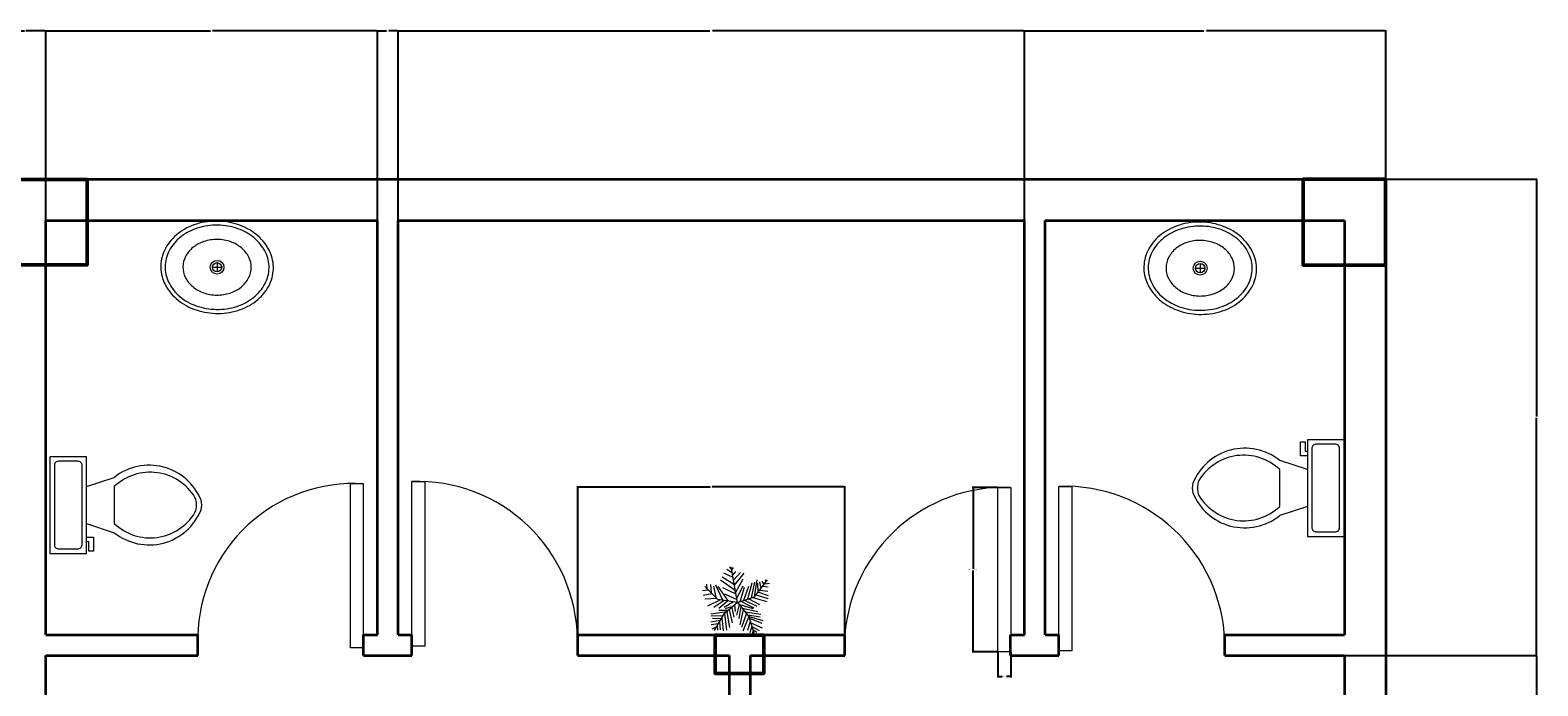
# Model space of a CAD drawing. Units: inches. Extents: x 50 to 2003, y -28 to 675.
# Tile 4 of 10: x 218 to 545, y 532 to 675. Entities that reach past the tile are written whole.
import ezdxf

# ---------------------------------------------------------------- set-up
doc = ezdxf.new("R2010")
doc.units = ezdxf.units.IN
for name, color, linetype, lineweight in [('A-ANNO-DIMS', 2, 'Continuous', 18), ('A-COLS', 1, 'Continuous', 50), ('A-DOOR', 4, 'Continuous', 18), ('A-FLOR-FIXT', 9, 'Continuous', 18), ('A-WALL', 7, 'Continuous', 35), ('L-PLNT', 3, 'Continuous', 13)]:
    doc.layers.add(name, color=color, linetype=linetype, lineweight=lineweight)
doc.styles.get("Standard").update_dxf_attribs({"font": 'arial.ttf'})
doc.dimstyles.get("Standard").update_dxf_attribs({"dimtxt": 0.18, "dimasz": 0.18, "dimexe": 0.18, "dimexo": 0.0625, "dimgap": 0.09, "dimtad": 0, "dimtih": 1, "dimtoh": 1, "dimdec": 4, "dimzin": 0, "dimdsep": 46, "dimtxsty": 'Standard', "dimcen": 0.09, "dimadec": 0, "dimazin": 0, "dimtfac": 1, "dimtdec": 4, "dimtofl": 0, "dimtmove": 0, "dimatfit": 3, "dimfxl": 1, "dimtolj": 1, "dimtzin": 0, "dimarcsym": 0})

# ---------------------------------------------------------------- blocks, each defined once
blk = doc.blocks.new('*U2')
for p, q in [((-8.737, 47.138), (-17.069, 52.711)), ((-10.186, 53.64), (-13.084, 55.962)), ((0, 0), (-10.5, 57)), ((-9.099, 51.782), (-6.563, 55.962)), ((-7.65, 43.423), (-2.578, 49.46)), ((-31.5, 4.5), (-52.5, 25.5)), ((-48.585, 21.131), (-49.309, 29.026)), ((-43.513, 28.561), (-42.427, 15.558)), ((-38.442, 26.239), (-34.819, 7.663)), ((-35.544, 28.097), (-24.314, 3.947)), ((-14.533, 2.09), (-30.834, 25.31)), ((-3.665, 19.273), (-27.574, 35.527)), ((-5.114, 28.097), (-24.676, 40.636)), ((-7.288, 39.707), (-21.778, 46.673)), ((-5.839, 35.992), (4.667, 48.067)), ((-5.114, 27.632), (10.463, 46.673)), ((-2.941, 16.486), (8.652, 37.85)), ((-1.129, 6.734), (9.014, 26.704)), ((3.942, 1.625), (11.187, 24.381)), ((10.101, 3.483), (17.708, 26.239)), ((16.259, 5.805), (23.142, 31.348)), ((22.055, 7.198), (27.489, 32.277)), ((27, 9), (48, 36)), ((27.127, 9.056), (31.112, 35.992)), ((31.836, 30.883), (32.561, 16.486)), ((35.096, 32.741), (37.27, 22.524)), ((38.719, 34.134), (41.979, 28.561)), ((40.53, 25.775), (48.862, 24.846)), ((43.791, 29.954), (51.036, 30.883)), ((44.153, 36.456), (45.239, 32.741)), ((-47.498, 19.737), (-55.83, 18.344)), ((-40.615, 13.7), (-55.105, 10.913)), ((-33.37, 6.269), (-52.207, 5.34)), ((-28.299, 3.483), (-47.86, -5.805)), ((-21.416, 3.018), (-38.079, -8.128)), ((0, 0), (-31.5, 4.5)), ((-15.982, 2.09), (-30.11, -9.521)), ((-24.314, 23.917), (-2.941, 13.7)), ((0, 0), (-22.5, -19.5)), ((-6.563, 1.161), (-21.416, -8.128)), ((-20.691, 13.7), (-1.129, 4.876)), ((0, 0), (27, 9)), ((0, 0), (18, -22.5)), ((6.478, 1.625), (26.04, -8.592)), ((11.187, 3.483), (30.749, -5.805)), ((18.07, 5.805), (35.096, -3.483)), ((24.229, 7.663), (46.688, 1.625)), ((29.662, 12.307), (48.137, 6.269)), ((33.285, 16.486), (48.862, 10.913)), ((36.183, 19.737), (48.137, 17.88)), ((-17.431, -15.094), (-42.789, -18.809)), ((-24.314, -21.596), (-42.427, -22.06)), ((-22.5, -19.5), (-37.5, -45)), ((-15.257, -12.772), (-30.11, -12.772)), ((-25.038, -23.918), (-22.865, -45.281)), ((-20.691, -18.345), (-17.793, -44.352)), ((-6.563, -5.805), (-19.967, -9.985)), ((-17.069, -15.094), (-12.721, -40.172)), ((-13.446, -11.378), (-8.737, -32.741)), ((-9.461, -8.592), (-6.201, -23.453)), ((-4.752, -3.483), (-3.665, -14.629)), ((2.493, -3.019), (-1.491, -20.202)), ((1.769, -2.555), (24.229, -9.521)), ((5.029, -6.27), (2.131, -25.775)), ((9.014, -11.378), (3.58, -35.992)), ((14.085, -16.951), (6.478, -40.172)), ((7.565, -9.056), (32.198, -14.629)), ((18.07, -22.524), (8.289, -45.745)), ((12.274, -15.094), (36.907, -18.809)), ((16.259, -19.738), (36.183, -22.989)), ((18, -22.5), (27, -52.5)), ((18.433, -22.524), (40.53, -29.026)), ((-28.299, -29.026), (-42.789, -31.348)), ((-30.834, -34.135), (-42.427, -35.528)), ((-34.457, -39.708), (-40.978, -42.494)), ((-26.849, -26.24), (-40.253, -25.775)), ((-32.646, -36.921), (-31.921, -44.352)), ((-29.023, -30.884), (-27.936, -43.887)), ((20.244, -30.419), (15.897, -44.816)), ((19.157, -25.311), (38.719, -33.206)), ((22.78, -37.85), (19.519, -48.532)), ((21.331, -32.741), (39.081, -40.636)), ((22.78, -38.314), (34.372, -44.816)), ((24.591, -45.745), (23.142, -50.854)), ((24.591, -43.423), (30.749, -47.603)), ((26.764, -49.925), (28.213, -50.854))]:
    blk.add_line(p, q)
blk = doc.blocks.new('Toilet - top')
for p, q in [((9.5, -6), (9.5, -2)), ((-10, -8.5), (-8, -8.5)), ((-10, -9.5), (-10, -8.5)), ((-7, -9.5), (-10, -9.5)), ((-8, -8.5), (-8, -8)), ((-7, -8), (-7, -9.5)), ((-4, -8), (-6, -14)), ((4, -8), (6, -14)), ((4, -14), (-4, -14))]:
    blk.add_line(p, q)
blk.add_lwpolyline([(10.5, -8), (10.5, 0), (-10.5, 0), (-10.5, -8)], close=True)
for points in [[(-9.5, -2), (-9.5, -6)], [(8.5, -1), (-8.5, -1)], [(-8.5, -7), (8.5, -7)]]:
    blk.add_lwpolyline(points)
for centre, radius, start, end in [((-8.62, -1.88), 0.884, 81.8699, 188.1301), ((8.62, -1.88), 0.884, 351.8699, 98.1301), ((-8.62, -6.12), 0.884, 171.8699, 278.1301), ((8.62, -6.12), 0.884, 261.8699, 8.1301), ((3.52, -21.58), 12.17, 141.4691, 247.9714), ((4.2, -21.82), 11.33, 136.3677, 238.9468), ((-3.52, -21.58), 12.17, 292.0284, 38.5307), ((-4.2, -21.82), 11.33, 301.053, 43.6321), ((0, -27.88), 4, 245.7318, 294.2682), ((0, -29), 4, 254.8605, 285.1395)]:
    blk.add_arc(centre, radius, start, end)
blk = doc.blocks.new('Sink - Oval top')
for p, q in [((-1, 0), (1, 0)), ((0, 1), (0, -1))]:
    blk.add_line(p, q)
for points in [[(-12.23, 0.39, 0.117634), (-11.46, -3.36, 0.104469), (-8.88, -6.8, 0.090016), (-5.08, -9.07, 0.08192), (-0.32, -10.02, 0.08192), (4.49, -9.38, 0.090016), (8.42, -7.36, 0.104469), (11.22, -4.09, 0.117634), (12.23, -0.39, 0.117634), (11.46, 3.36, 0.104469), (8.88, 6.8, 0.090016), (5.08, 9.07, 0.08192), (0.32, 10.02, 0.08192), (-4.49, 9.38, 0.090016), (-8.42, 7.36, 0.104469), (-11.22, 4.09, 0.117634)], [(-11.29, 0.16, 0.118622), (-10.52, -3.25, 0.104678), (-8.07, -6.36, 0.089562), (-4.54, -8.37, 0.081185), (-0.13, -9.15, 0.081185), (4.3, -8.49, 0.089562), (7.89, -6.58, 0.104678), (10.42, -3.55, 0.118622), (11.29, -0.16, 0.118622), (10.52, 3.25, 0.104678), (8.07, 6.36, 0.089562), (4.54, 8.37, 0.081185), (0.13, 9.15, 0.081185), (-4.3, 8.49, 0.089562), (-7.89, 6.58, 0.104678), (-10.42, 3.55, 0.118622)], [(-7.42, 0.08, 0.118283), (-6.91, -2.17, 0.104607), (-5.29, -4.21, 0.089718), (-2.97, -5.53, 0.081436), (-0.07, -6.04, 0.081436), (2.84, -5.59, 0.089718), (5.2, -4.33, 0.104607), (6.86, -2.32, 0.118283), (7.42, -0.08, 0.118283), (6.91, 2.17, 0.104607), (5.29, 4.21, 0.089718), (2.97, 5.53, 0.081436), (0.07, 6.04, 0.081436), (-2.84, 5.59, 0.089718), (-5.2, 4.33, 0.104607), (-6.86, 2.32, 0.118283)]]:
    blk.add_lwpolyline(points, format="xyb", close=True)
for radius in [1.5, 1]:
    blk.add_circle((0, 0), radius)
blk = doc.blocks.new('DOOR-LEAF-36')
blk.add_lwpolyline([(35.71, 2.81), (35.71, 0), (0, 0), (0, 2.81)], close=True)
blk = doc.blocks.new('*D21')
at = {"layer": 'A-ANNO-DIMS', "color": 0, "lineweight": -2, "transparency": 16777216}
for p, q in [((427.62, 575.33), (422.15, 575.33)), ((422.33, 575.15), (422.33, 557.66)), ((422.33, 539.81), (422.33, 557.3)), ((427.62, 539.63), (422.15, 539.63))]:
    blk.add_line(p, q, dxfattribs=at)
at = {"layer": 'A-ANNO-DIMS', "color": 0, "transparency": 16777216}
for points in [[(422.3, 575.15), (422.36, 575.15), (422.33, 575.33)], [(422.3, 539.81), (422.36, 539.81), (422.33, 539.63)]]:
    blk.add_solid(points, dxfattribs=at)
at = {"layer": 'Defpoints', "color": 0, "transparency": 16777216}
for p in [(427.69, 575.33), (422.33, 539.63), (427.69, 539.63)]:
    blk.add_point(p, dxfattribs=at)
at = {"layer": 'A-ANNO-DIMS', "color": 0, "transparency": 16777216, "insert": (422.33, 557.48), "char_height": 0.18, "attachment_point": 5}
blk.add_mtext('\\A1;DOOR LEAF 36 TYP.', dxfattribs=at)
blk = doc.blocks.new('*D22')
at = {"layer": 'A-ANNO-DIMS', "color": 0, "lineweight": -2, "transparency": 16777216}
for p, q in [((427.69, 539.56), (427.69, 534.09)), ((430.5, 539.56), (430.5, 534.09)), ((427.87, 534.27), (428.63, 534.27)), ((430.32, 534.27), (429.55, 534.27))]:
    blk.add_line(p, q, dxfattribs=at)
at = {"layer": 'A-ANNO-DIMS', "color": 0, "transparency": 16777216}
for points in [[(427.87, 534.3), (427.87, 534.24), (427.69, 534.27)], [(430.32, 534.3), (430.32, 534.24), (430.5, 534.27)]]:
    blk.add_solid(points, dxfattribs=at)
at = {"layer": 'Defpoints', "color": 0, "transparency": 16777216}
for p in [(427.69, 539.63), (430.5, 539.63), (430.5, 534.27)]:
    blk.add_point(p, dxfattribs=at)
at = {"layer": 'A-ANNO-DIMS', "color": 0, "transparency": 16777216, "insert": (429.09, 534.27), "char_height": 0.18, "attachment_point": 5}
blk.add_mtext('\\A1;3 TYP.', dxfattribs=at)
blk = doc.blocks.new('*D54')
at = {"layer": 'A-ANNO-DIMS', "color": 0, "lineweight": -2, "transparency": 16777216}
for p, q in [((211.97, 642.39), (211.97, 674.65)), ((212.15, 674.47), (216.32, 674.47)), ((220.79, 674.47), (216.62, 674.47)), ((220.97, 633.39), (220.97, 674.65))]:
    blk.add_line(p, q, dxfattribs=at)
at = {"layer": 'A-ANNO-DIMS', "color": 0, "transparency": 16777216}
for points in [[(212.15, 674.5), (212.15, 674.44), (211.97, 674.47)], [(220.79, 674.5), (220.79, 674.44), (220.97, 674.47)]]:
    blk.add_solid(points, dxfattribs=at)
at = {"layer": 'Defpoints', "color": 0, "transparency": 16777216}
for p in [(220.97, 674.47), (211.97, 642.32), (220.97, 633.32)]:
    blk.add_point(p, dxfattribs=at)
at = {"layer": 'A-ANNO-DIMS', "color": 0, "transparency": 16777216, "insert": (216.47, 674.47), "char_height": 0.18, "attachment_point": 5}
blk.add_mtext('\\A1;9', dxfattribs=at)
blk = doc.blocks.new('*D55')
at = {"layer": 'A-ANNO-DIMS', "color": 0, "lineweight": -2, "transparency": 16777216}
for p, q in [((220.97, 633.39), (220.97, 674.65)), ((221.15, 674.47), (256.75, 674.47)), ((292.79, 674.47), (257.19, 674.47)), ((292.97, 633.39), (292.97, 674.65))]:
    blk.add_line(p, q, dxfattribs=at)
at = {"layer": 'A-ANNO-DIMS', "color": 0, "transparency": 16777216}
for points in [[(221.15, 674.5), (221.15, 674.44), (220.97, 674.47)], [(292.79, 674.5), (292.79, 674.44), (292.97, 674.47)]]:
    blk.add_solid(points, dxfattribs=at)
at = {"layer": 'Defpoints', "color": 0, "transparency": 16777216}
for p in [(292.97, 674.47), (220.97, 633.32), (292.97, 633.32)]:
    blk.add_point(p, dxfattribs=at)
at = {"layer": 'A-ANNO-DIMS', "color": 0, "transparency": 16777216, "insert": (256.97, 674.47), "char_height": 0.18, "attachment_point": 5}
blk.add_mtext('\\A1;72', dxfattribs=at)
blk = doc.blocks.new('*D56')
at = {"layer": 'A-ANNO-DIMS', "color": 0, "lineweight": -2, "transparency": 16777216}
for p, q in [((292.97, 633.39), (292.97, 674.65)), ((293.15, 674.47), (294.96, 674.47)), ((297.29, 674.47), (295.48, 674.47)), ((297.47, 633.39), (297.47, 674.65))]:
    blk.add_line(p, q, dxfattribs=at)
at = {"layer": 'A-ANNO-DIMS', "color": 0, "transparency": 16777216}
for points in [[(293.15, 674.5), (293.15, 674.44), (292.97, 674.47)], [(297.29, 674.5), (297.29, 674.44), (297.47, 674.47)]]:
    blk.add_solid(points, dxfattribs=at)
at = {"layer": 'Defpoints', "color": 0, "transparency": 16777216}
for p in [(297.47, 674.47), (292.97, 633.32), (297.47, 633.32)]:
    blk.add_point(p, dxfattribs=at)
at = {"layer": 'A-ANNO-DIMS', "color": 0, "transparency": 16777216, "insert": (295.22, 674.47), "char_height": 0.18, "attachment_point": 5}
blk.add_mtext('\\A1;4.5', dxfattribs=at)
blk = doc.blocks.new('*D57')
at = {"layer": 'A-ANNO-DIMS', "color": 0, "lineweight": -2, "transparency": 16777216}
for p, q in [((297.47, 633.39), (297.47, 674.65)), ((297.65, 674.47), (365.19, 674.47)), ((433.29, 674.47), (365.75, 674.47)), ((433.47, 633.39), (433.47, 674.65))]:
    blk.add_line(p, q, dxfattribs=at)
at = {"layer": 'A-ANNO-DIMS', "color": 0, "transparency": 16777216}
for points in [[(297.65, 674.5), (297.65, 674.44), (297.47, 674.47)], [(433.29, 674.5), (433.29, 674.44), (433.47, 674.47)]]:
    blk.add_solid(points, dxfattribs=at)
at = {"layer": 'Defpoints', "color": 0, "transparency": 16777216}
for p in [(433.47, 674.47), (297.47, 633.32), (433.47, 633.32)]:
    blk.add_point(p, dxfattribs=at)
at = {"layer": 'A-ANNO-DIMS', "color": 0, "transparency": 16777216, "insert": (365.47, 674.47), "char_height": 0.18, "attachment_point": 5}
blk.add_mtext('\\A1;136', dxfattribs=at)
blk = doc.blocks.new('*D58')
at = {"layer": 'A-ANNO-DIMS', "color": 0, "lineweight": -2, "transparency": 16777216}
for p, q in [((433.47, 633.39), (433.47, 674.65)), ((433.65, 674.47), (472.4, 674.47)), ((511.79, 674.47), (473.04, 674.47)), ((511.97, 642.39), (511.97, 674.65))]:
    blk.add_line(p, q, dxfattribs=at)
at = {"layer": 'A-ANNO-DIMS', "color": 0, "transparency": 16777216}
for points in [[(433.65, 674.5), (433.65, 674.44), (433.47, 674.47)], [(511.79, 674.5), (511.79, 674.44), (511.97, 674.47)]]:
    blk.add_solid(points, dxfattribs=at)
at = {"layer": 'Defpoints', "color": 0, "transparency": 16777216}
for p in [(511.97, 674.47), (511.97, 642.32), (433.47, 633.32)]:
    blk.add_point(p, dxfattribs=at)
at = {"layer": 'A-ANNO-DIMS', "color": 0, "transparency": 16777216, "insert": (472.72, 674.47), "char_height": 0.18, "attachment_point": 5}
blk.add_mtext('\\A1;78.5', dxfattribs=at)
blk = doc.blocks.new('*D62')
at = {"layer": 'A-ANNO-DIMS', "color": 0, "lineweight": -2, "transparency": 16777216}
for p, q in [((503.03, 538.82), (544.84, 538.82)), ((544.66, 538.64), (544.66, 465.26)), ((544.66, 391.5), (544.66, 464.89)), ((503.03, 391.32), (544.84, 391.32))]:
    blk.add_line(p, q, dxfattribs=at)
at = {"layer": 'A-ANNO-DIMS', "color": 0, "transparency": 16777216}
for points in [[(544.63, 538.64), (544.69, 538.64), (544.66, 538.82)], [(544.63, 391.5), (544.69, 391.5), (544.66, 391.32)]]:
    blk.add_solid(points, dxfattribs=at)
at = {"layer": 'Defpoints', "color": 0, "transparency": 16777216}
for p in [(502.97, 538.82), (544.66, 538.82), (502.97, 391.32)]:
    blk.add_point(p, dxfattribs=at)
at = {"layer": 'A-ANNO-DIMS', "color": 0, "transparency": 16777216, "insert": (544.66, 465.07), "char_height": 0.18, "attachment_point": 5}
blk.add_mtext('\\A1;147.5', dxfattribs=at)
blk = doc.blocks.new('*D63')
at = {"layer": 'A-ANNO-DIMS', "color": 0, "lineweight": -2, "transparency": 16777216}
for p, q in [((512.03, 642.32), (544.84, 642.32)), ((544.66, 642.14), (544.66, 590.76)), ((544.66, 539), (544.66, 590.39)), ((503.03, 538.82), (544.84, 538.82))]:
    blk.add_line(p, q, dxfattribs=at)
at = {"layer": 'A-ANNO-DIMS', "color": 0, "transparency": 16777216}
for points in [[(544.63, 642.14), (544.69, 642.14), (544.66, 642.32)], [(544.63, 539), (544.69, 539), (544.66, 538.82)]]:
    blk.add_solid(points, dxfattribs=at)
at = {"layer": 'Defpoints', "color": 0, "transparency": 16777216}
for p in [(511.97, 642.32), (544.66, 642.32), (502.97, 538.82)]:
    blk.add_point(p, dxfattribs=at)
at = {"layer": 'A-ANNO-DIMS', "color": 0, "transparency": 16777216, "insert": (544.66, 590.57), "char_height": 0.18, "attachment_point": 5}
blk.add_mtext('\\A1;103.5', dxfattribs=at)
blk = doc.blocks.new('*D69')
at = {"layer": 'A-ANNO-DIMS', "color": 0, "lineweight": -2, "transparency": 16777216}
for p, q in [((336.47, 543.39), (336.47, 575.65)), ((336.65, 575.47), (365.25, 575.47)), ((394.29, 575.47), (365.69, 575.47)), ((394.47, 543.39), (394.47, 575.65))]:
    blk.add_line(p, q, dxfattribs=at)
at = {"layer": 'A-ANNO-DIMS', "color": 0, "transparency": 16777216}
for points in [[(336.65, 575.5), (336.65, 575.44), (336.47, 575.47)], [(394.29, 575.5), (394.29, 575.44), (394.47, 575.47)]]:
    blk.add_solid(points, dxfattribs=at)
at = {"layer": 'Defpoints', "color": 0, "transparency": 16777216}
for p in [(394.47, 575.47), (336.47, 543.32), (394.47, 543.32)]:
    blk.add_point(p, dxfattribs=at)
at = {"layer": 'A-ANNO-DIMS', "color": 0, "transparency": 16777216, "insert": (365.47, 575.47), "char_height": 0.18, "attachment_point": 5}
blk.add_mtext('\\A1;58', dxfattribs=at)

msp = doc.modelspace()

# ---------------------------------------------------------------- linework, layer by layer
at = {"layer": 'A-COLS'}
for points in [[(211.9898, 642.1898), (229.9336, 642.1898), (229.9336, 623.6596), (211.9898, 623.6596)], [(511.9071, 642.2546), (493.9902, 642.2546), (493.9902, 623.6344), (511.9071, 623.6344)], [(366.2895, 543.2564), (376.8583, 543.2564), (376.8583, 534.9486), (366.2895, 534.9486)]]:
    msp.add_lwpolyline(points, close=True, dxfattribs=at)
at = {"layer": 'A-DOOR'}
for centre, radius, start, end in [((287.8796, 542.2862), 33.9113, 86.591193, 178.879605), ((301.7332, 541.9614), 34.669, 0.787409, 92.068961), ((429.1629, 540.5706), 34.7894, 87.826126, 175.644292), ((442.1372, 540.7332), 34.8536, 1.948939, 91.91482)]:
    msp.add_arc(centre, radius, start, end, dxfattribs=at)
at = {"layer": 'A-WALL'}
for p, q in [((211.9711, 642.3232), (511.9711, 642.3232)), ((511.9711, 642.3232), (511.9711, 17.3232)), ((220.9711, 633.3232), (292.9711, 633.3232)), ((220.9711, 543.3232), (220.9711, 633.3232)), ((292.9711, 543.3232), (292.9711, 633.3232)), ((297.4711, 543.3232), (297.4711, 633.3232)), ((297.4711, 633.3232), (433.4711, 633.3232)), ((433.4711, 543.3232), (433.4711, 633.3232)), ((437.9711, 543.3232), (437.9711, 633.3232)), ((437.9711, 633.3232), (502.9711, 633.3232)), ((502.9711, 633.3232), (502.9711, 543.3232)), ((220.9711, 543.3232), (253.9711, 543.3232)), ((253.9711, 538.8232), (253.9711, 543.3232)), ((289.9711, 538.8232), (289.9711, 543.3232)), ((289.9711, 543.3232), (292.9711, 543.3232)), ((297.4711, 543.3232), (300.4711, 543.3232)), ((300.4711, 538.8232), (300.4711, 543.3232)), ((336.4711, 538.8232), (336.4711, 543.3232)), ((336.4711, 543.3232), (394.4711, 543.3232)), ((394.4711, 538.8232), (394.4711, 543.3232)), ((430.4711, 538.8232), (430.4711, 543.3232)), ((430.4711, 543.3232), (433.4711, 543.3232)), ((437.9711, 543.3232), (440.9711, 543.3232)), ((440.9711, 538.8232), (440.9711, 543.3232)), ((476.9711, 538.8232), (476.9711, 543.3232)), ((476.9711, 543.3232), (502.9711, 543.3232)), ((220.9711, 538.8232), (253.9711, 538.8232)), ((220.9711, 395.8232), (220.9711, 538.8232)), ((289.9711, 538.8232), (300.4711, 538.8232)), ((336.4711, 538.8232), (369.4711, 538.8232)), ((369.4711, 395.8232), (369.4711, 538.8232)), ((373.9711, 395.8232), (373.9711, 538.8232)), ((373.9711, 538.8232), (394.4711, 538.8232)), ((430.4711, 538.8232), (440.9711, 538.8232)), ((476.9711, 538.8232), (502.9711, 538.8232)), ((502.9711, 538.8232), (502.9711, 395.8232))]:
    msp.add_line(p, q, dxfattribs=at)

# ---------------------------------------------------------------- block references
at = {"layer": 'A-DOOR'}
for p, rotation in [((300.4835, 576.6088), 269.9999999999999), ((287.1102, 576.1839), 269.9999999999999), ((427.6868, 575.3339), 269.9999999999998), ((440.9775, 575.5669), 269.9999999999998)]:
    msp.add_blockref('DOOR-LEAF-36', p, dxfattribs=dict(at, rotation=rotation))
at = {"layer": 'A-FLOR-FIXT'}
for p in [(258.1642, 623.1544), (471.6425, 622.9522)]:
    msp.add_blockref('Sink - Oval top', p, dxfattribs=at)
for p, rotation in [((502.9091, 575.2126), 270), ((221.8432, 571.5115), 89.99999999999999)]:
    msp.add_blockref('Toilet - top', p, dxfattribs=dict(at, rotation=rotation))
at = {"layer": 'L-PLNT', "xscale": 0.1358686367750108, "yscale": 0.1358686367750108, "zscale": 0.1358686367750108}
msp.add_blockref('*U2', (371.192, 550.3577), dxfattribs=at)

# ---------------------------------------------------------------- dimensions: what is measured, and where the dimension line sits
at = {"layer": 'A-ANNO-DIMS'}
for base, p1, p2, override, picture, middle in [((220.9711, 674.4732), (211.9711, 642.3232), (220.9711, 633.3232), {"dimdec": 0, "dimlfac": 1, "dimrnd": 0, "dimzin": 0, "dimdsep": 46, "dimlunit": 2}, '*D54', (216.4711, 674.4732)), ((292.9711, 674.4732), (220.9711, 633.3232), (292.9711, 633.3232), {"dimdec": 0, "dimlfac": 1, "dimrnd": 0, "dimzin": 0, "dimdsep": 46, "dimlunit": 2}, '*D55', (256.9711, 674.4732)), ((297.4711, 674.4732), (292.9711, 633.3232), (297.4711, 633.3232), {"dimdec": 1, "dimlfac": 1, "dimrnd": 0, "dimzin": 0, "dimdsep": 46, "dimlunit": 2}, '*D56', (295.2211, 674.4732)), ((433.4711, 674.4732), (297.4711, 633.3232), (433.4711, 633.3232), {"dimdec": 0, "dimlfac": 1, "dimrnd": 0, "dimzin": 0, "dimdsep": 46, "dimlunit": 2}, '*D57', (365.4711, 674.4732)), ((511.9711, 674.4732), (433.4711, 633.3232), (511.9711, 642.3232), {"dimdec": 1, "dimlfac": 1, "dimrnd": 0, "dimzin": 0, "dimdsep": 46, "dimlunit": 2}, '*D58', (472.7211, 674.4732)), ((394.4711, 575.4732), (336.4711, 543.3232), (394.4711, 543.3232), {"dimdec": 0, "dimlfac": 1, "dimrnd": 0, "dimzin": 0, "dimdsep": 46, "dimlunit": 2}, '*D69', (365.4711, 575.4732))]:
    dim = msp.add_linear_dim(base=base, p1=p1, p2=p2, dimstyle='Standard', override=override, dxfattribs=at)
    dim.commit()
    dim.dimension.update_dxf_attribs({"geometry": picture, "text_midpoint": middle})
for base, p1, p2, picture, middle in [((544.6551, 642.3232), (502.9711, 538.8232), (511.9711, 642.3232), '*D63', (544.6551, 590.5732)), ((544.6551, 538.8232), (502.9711, 391.3232), (502.9711, 538.8232), '*D62', (544.6551, 465.0732))]:
    dim = msp.add_linear_dim(base=base, p1=p1, p2=p2, angle=90, dimstyle='Standard', override={"dimdec": 1, "dimlfac": 1, "dimrnd": 0, "dimzin": 0, "dimdsep": 46, "dimlunit": 2}, dxfattribs=at)
    dim.commit()
    dim.dimension.update_dxf_attribs({"geometry": picture, "text_midpoint": middle})
dim = msp.add_linear_dim(base=(422.3306, 539.6263), p1=(427.6868, 575.3339), p2=(427.6868, 539.6263), angle=270, text='DOOR LEAF <> TYP.', dimstyle='Standard', override={"dimdec": 0, "dimlfac": 1, "dimrnd": 0, "dimzin": 0, "dimdsep": 46, "dimlunit": 2}, dxfattribs=at)
dim.commit()
dim.dimension.update_dxf_attribs({"geometry": '*D21', "text_midpoint": (422.3306, 557.4801)})
dim = msp.add_linear_dim(base=(430.497, 534.2702), p1=(427.6868, 539.6263), p2=(430.497, 539.6263), text='<> TYP.', dimstyle='Standard', override={"dimdec": 0, "dimlfac": 1, "dimrnd": 0, "dimzin": 0, "dimdsep": 46, "dimlunit": 2}, dxfattribs=at)
dim.commit()
dim.dimension.update_dxf_attribs({"geometry": '*D22', "text_midpoint": (429.0919, 534.2702)})

doc.saveas('drawing.dxf')
